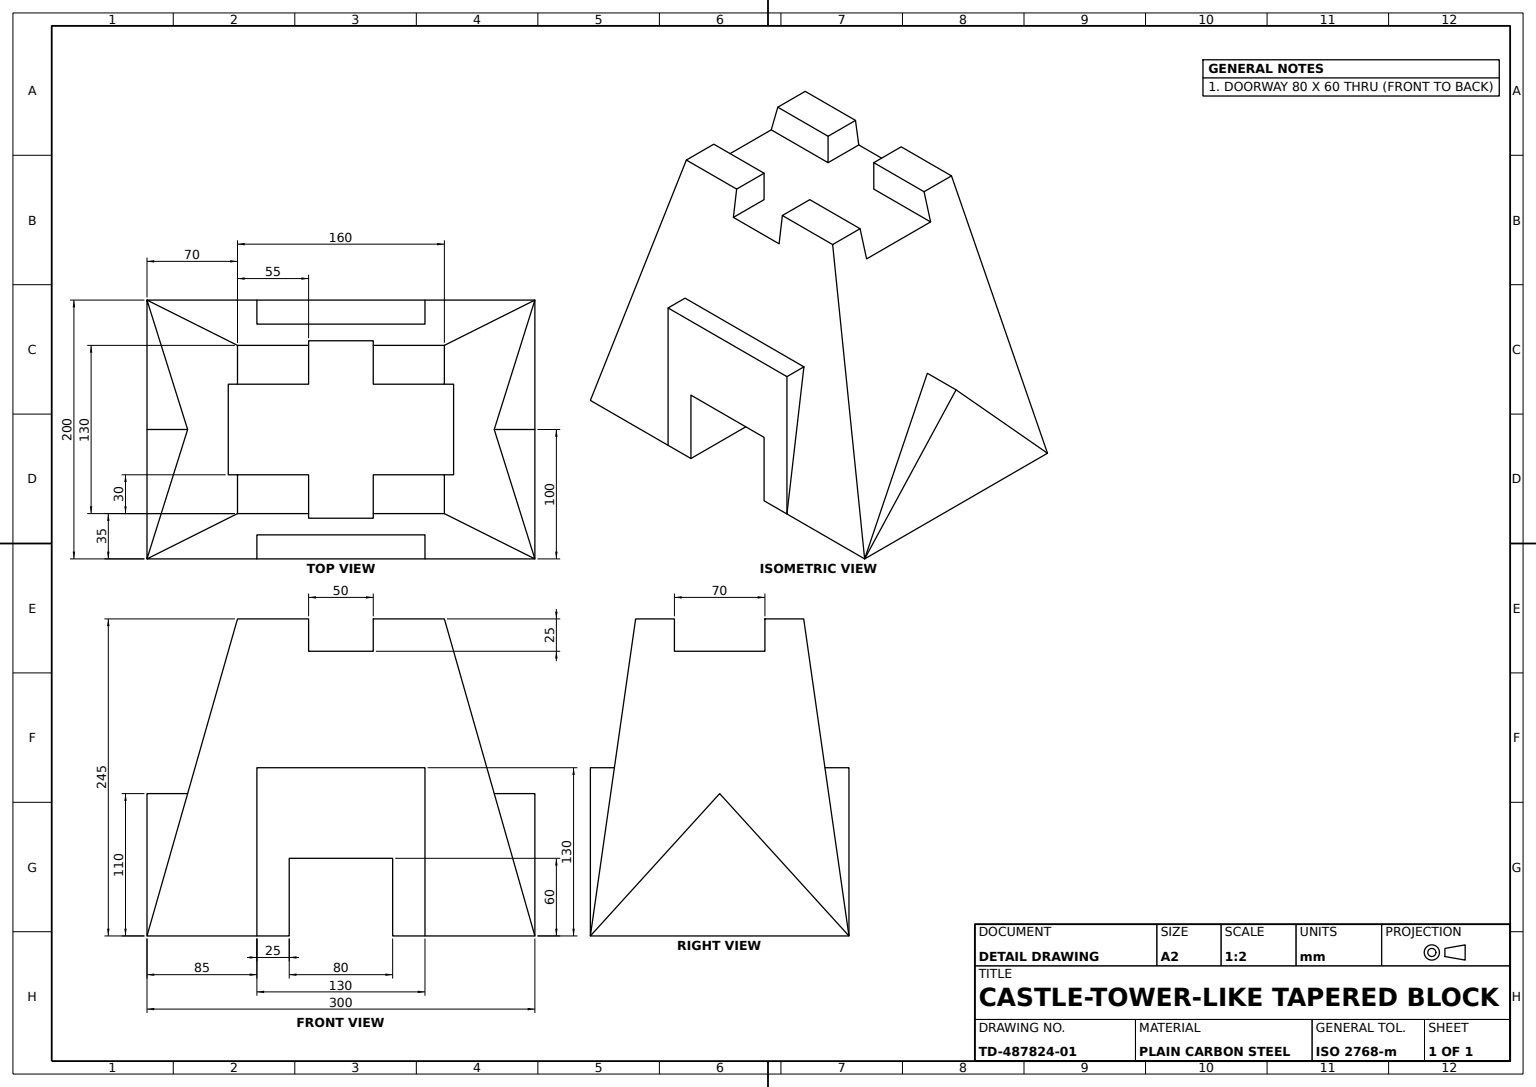
SolidWorks part; units mm, degrees
material "Plain Carbon Steel"
ref_plane "Front Plane" through (0, 0, 0) normal (0, 0, 1) x (1, 0, 0)
ref_plane "Top Plane" through (0, 0, 0) normal (0, 1, 0) x (1, 0, 0)
ref_plane "Right Plane" through (0, 0, 0) normal (1, 0, 0) x (0, 0, -1)
sketch "Base Profile 300x200" plane through (0, 0, 0) normal (0, 1, 0) x (1, 0, 0)
  line L1 (-150, -100) -> (150, -100)
  line L2 (-150, -100) -> (-150, 100)
  line L3 (-150, 100) -> (150, 100)
  line L4 (150, -100) -> (150, 100)
  line L5 (-150, -100) -> (150, 100) construction
  line L6 (-150, 100) -> (150, -100) construction
  point P0 (0, 0)
  dimension "D1" = 200
  dimension "D2" = 300
ref_plane "Top Profile Plane" through (0, 245, 0) normal (0, 1, 0) x (1, 0, 0)
sketch "Top Profile 160x130" plane through (0, 245, 0) normal (0, 1, 0) x (1, 0, 0)
  line L1 (-80, -65) -> (80, -65)
  line L2 (-80, -65) -> (-80, 65)
  line L3 (-80, 65) -> (80, 65)
  line L4 (80, -65) -> (80, 65)
  line L5 (-80, -65) -> (80, 65) construction
  line L6 (-80, 65) -> (80, -65) construction
  point P0 (0, 0)
  dimension "D1" = 130
  dimension "D2" = 160
loft "Pyramidal Body Loft" add profiles "Top Profile 160x130", "Base Profile 300x200"
sketch "Gate Block Profile 130x130" plane through (0, 0, 0) normal (0, 0, 1) x (1, 0, 0)
  line L0 (-65, 0) -> (-65, 130)
  line L1 (-150, 0) -> (150, 0) construction
  line L2 (-65, 130) -> (65, 130)
  line L3 (65, 130) -> (65, 0)
  line L4 (-65, 0) -> (65, 0)
  point P4 (0, 130)
  dimension "D1" = 130
  dimension "D2" = 130
extrude "Gate Block" add sketch "Gate Block Profile 130x130" along normal mid plane 200
sketch "Side Buttress Profile" plane through (0, 0, 0) normal (1, 0, 0) x (0, 0, -1)
  line L0 (-100, 0) -> (0, 110)
  line L1 (0, 110) -> (100, 0)
  line L2 (-100, 0) -> (100, 0) construction
  line L3 (-100, 0) -> (100, 0)
  dimension "D1" = 110
extrude "Side Buttress" add sketch "Side Buttress Profile" along normal mid plane 300
sketch "Doorway Profile 60x80" plane through (0, 0, 0) normal (0, 0, 1) x (1, 0, 0)
  line L0 (-65, 0) -> (65, 0) construction
  line L1 (-40, 0) -> (40, 0)
  line L2 (-40, 0) -> (-40, 60)
  line L3 (-40, 60) -> (40, 60)
  line L4 (40, 0) -> (40, 60)
  point P6 (0, 60)
  dimension "D1" = 60
  dimension "D2" = 80
extrude "Doorway Cut" cut sketch "Doorway Profile 60x80" against normal through all both and the other way through all
sketch "Crenellation Profile" plane through (0, 245, 0) normal (0, 1, 0) x (1, 0, 0)
  line L0 (80, -65) -> (80, 65) construction
  line L1 (80, 65) -> (-80, 65) construction
  line L8 (-25, 65) -> (-25, 35)
  line L9 (-25, 35) -> (-80, 35)
  line L10 (0, 0) -> (0, 39.973) construction
  line L11 (0, 0) -> (-35.1179, 0) construction
  line L12 (25, 65) -> (25, 35)
  line L13 (25, 35) -> (80, 35)
  line L14 (-25, -35) -> (-80, -35)
  line L15 (-25, -65) -> (-25, -35)
  line L16 (25, -65) -> (25, -35)
  line L17 (25, -35) -> (80, -35)
  line L18 (-25, 65) -> (-25, 74.6054)
  line L19 (-25, 74.6054) -> (25, 74.6054)
  line L20 (25, 74.6054) -> (25, 65)
  line L21 (-80, 35) -> (-93.7989, 35)
  line L22 (-93.7989, 35) -> (-93.7989, -35)
  line L23 (-93.7989, -35) -> (-80, -35)
  line L24 (80, -35) -> (94.1873, -35)
  line L25 (94.1873, -35) -> (94.1873, 35)
  line L26 (94.1873, 35) -> (80, 35)
  line L27 (-25, -65) -> (-25, -87.9729)
  line L28 (-25, -87.9729) -> (25, -87.9729)
  line L29 (25, -87.9729) -> (25, -65)
  dimension "D1" = 14.1873
  dimension "D2" = 30
  dimension "D3" = 55
  dimension "D4" = 173.7989
  dimension "D5" = 160
  dimension "D6" = 9.6054
  dimension "D7" = 100
  dimension "D8" = 152.9729
extrude "Crenellation Cut 25 Deep" cut sketch "Crenellation Profile" against normal blind 25
